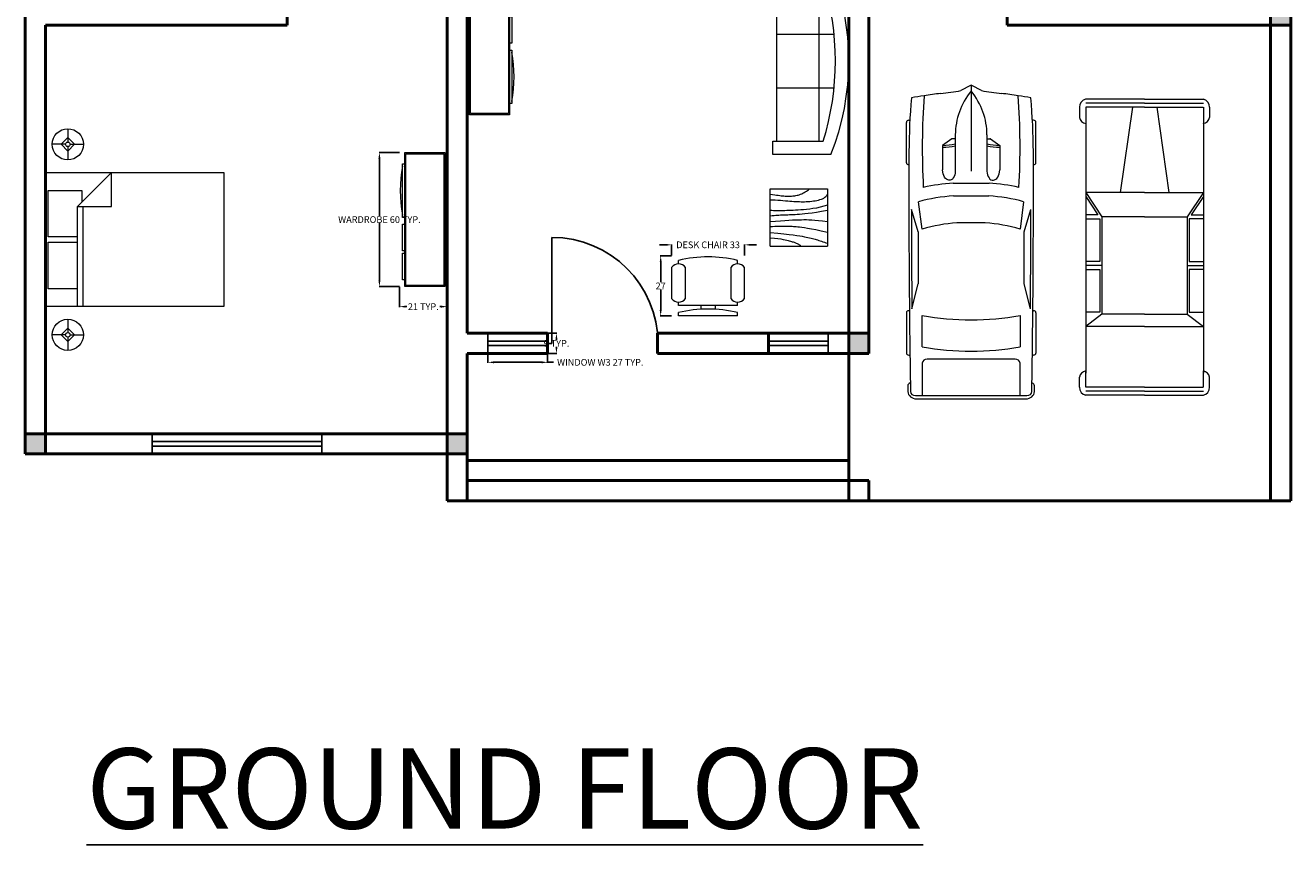
# Model space of a CAD drawing. Units: inches. Extents: x 13 to 1693, y -7 to 1519.
# Tile 1 of 10: x 116 to 683, y -7 to 360. Entities that reach past the tile are written whole.
import ezdxf

# ---------------------------------------------------------------- set-up
doc = ezdxf.new("R2010")
doc.units = ezdxf.units.IN
doc.header["$MEASUREMENT"] = 0
for name, color, linetype, lineweight in [('A-ANNO-DIMS', 2, 'Continuous', 18), ('A-ANNO-TEXT', 7, 'Continuous', 25), ('A-DOOR', 4, 'Continuous', 25), ('A-EQPM', 8, 'Continuous', 18), ('A-FURN', 8, 'Continuous', 18), ('A-GLAZ', 4, 'Continuous', 25), ('A-WALL', 7, 'Continuous', 50), ('A-WALL-PATT', 8, 'Continuous', 13)]:
    doc.layers.add(name, color=color, linetype=linetype, lineweight=lineweight)
doc.styles.get("Standard").update_dxf_attribs({"font": 'arial.ttf'})
doc.dimstyles.get("Standard").update_dxf_attribs({"dimtxt": 3, "dimasz": 2.68, "dimexe": 0.18, "dimexo": 0.0625, "dimgap": 0.09, "dimtad": 0, "dimtih": 1, "dimtoh": 1, "dimdec": 0, "dimzin": 0, "dimdsep": 46, "dimlunit": 3, "dimtxsty": 'Standard', "dimcen": 0.09, "dimadec": 0, "dimazin": 0, "dimtfac": 1, "dimtdec": 0, "dimtofl": 0, "dimtmove": 0, "dimatfit": 3, "dimfxl": 1, "dimtolj": 1, "dimtzin": 0, "dimarcsym": 0})

# ---------------------------------------------------------------- blocks, each defined once
blk = doc.blocks.new('Chair - Desk')
for p, q in [((-8.5, 0), (-8.5, -1)), ((-8.5, 0), (8.5, 0)), ((8.5, 0), (8.5, -1)), ((-8.5, -3), (-8.5, -4)), ((-8.5, -3), (8.5, -3)), ((-2, -3), (-2, -1.9355)), ((2, -1.9576), (2, -3)), ((8.5, -3), (8.5, -4)), ((-10.5, -5), (-10.5, -14)), ((-6.5, -14), (-6.5, -5)), ((6.5, -5), (6.5, -14)), ((10.5, -14), (10.5, -5)), ((-8.5, -15), (-8.5, -16)), ((8.5, -15), (8.5, -16))]:
    blk.add_line(p, q)
for centre, radius, start, end in [((0, 34.625), 36.625, 256.5803, 283.4197), ((-8.5, -6.5), 2.5, 36.8699, 143.1301), ((8.5, -6.5), 2.5, 36.8699, 143.1301), ((-8.5, -12.5), 2.5, 216.8699, 323.1301), ((8.5, -12.5), 2.5, 216.8699, 323.1301), ((0, 19.625), 36.625, 256.5803, 283.4197)]:
    blk.add_arc(centre, radius, start, end)
blk = doc.blocks.new('Sofa - Roundback 7 ft.')
for p, q in [((-12.00002, -32.4421), (-12.00003, -6.5971)), ((11.99997, -32.4421), (11.99998, -6.5971)), ((-36.000027, -34), (-36.000027, -11.4696)), ((-35.999844, -13.3819), (35.9998, -13.3819)), ((35.99998, -34), (35.99998, -11.4696)), ((-36.000027, -32.4421), (35.99998, -32.4421))]:
    blk.add_line(p, q)
for points in [[(-36.000027, -34), (-42.000027, -34), (-42.000027, -8)], [(41.99998, -8), (41.99998, -34), (35.99998, -34)]]:
    blk.add_lwpolyline(points)
for centre, radius, start, end in [((0, -114.25), 114.25, 68.43141, 111.5686), ((-0.00001, -127.1968), 121.1968, 72.72033, 107.2797)]:
    blk.add_arc(centre, radius, start, end)
blk = doc.blocks.new('Entertainment Center')
for p, q in [((-4, 0), (-5, -1)), ((4, 0), (-4, 0)), ((5, -1), (4, 0)), ((-17, -19), (-17, -1)), ((-17, -1), (43, -1)), ((-16.5, -18.5), (-16.5, -1.5)), ((-16.5, -1.5), (42.5, -1.5)), ((42.5, -1.5), (42.5, -18.5)), ((43, -1), (43, -19)), ((43, -19), (-17, -19)), ((42.5, -18.5), (-16.5, -18.5)), ((-12, -20), (-12, -19)), ((12, -20), (-12, -20)), ((12, -19), (12, -20)), ((15, -20), (15, -19)), ((27, -20), (15, -20)), ((27, -19), (27, -20)), ((28, -20), (28, -19)), ((40, -20), (28, -20)), ((40, -19), (40, -20))]:
    blk.add_line(p, q)
blk.add_arc((0, 40), 61, 259.6111, 280.3889)
blk = doc.blocks.new('Bed - Queen')
for p, q in [((0, -80.00003), (0, 0)), ((0, 0), (59.99999, 0)), ((59.99999, 0), (59.99999, -80.00003)), ((7.99999, -1.2), (28.79998, -1.2)), ((7.99999, -14.4), (7.99999, -1.2)), ((28.79998, -1.2), (28.79998, -14.4)), ((31.19999, -1.2), (51.99999, -1.2)), ((31.19999, -14.4), (31.19999, -1.2)), ((51.99999, -1.2), (51.99999, -16.4)), ((0, -14.4), (44.8, -14.4)), ((44.8, -16.8), (0, -16.8)), ((59.99999, -29.6), (44.8, -14.4)), ((44.8, -14.4), (44.8, -29.6)), ((51.99999, -16.4), (46.79936, -16.4)), ((44.8, -29.6), (59.99999, -29.6)), ((59.99999, -80.00003), (0, -80.00003))]:
    blk.add_line(p, q)
blk = doc.blocks.new('Lamp - Table')
for p, q in [((0, 7), (0, 1)), ((-1, 0), (-7, 0)), ((0, 3), (-3, 0)), ((-3, 0), (0, -3)), ((3, 0), (0, 3)), ((0, -3), (3, 0)), ((1, 0), (7, 0)), ((0, -1), (0, -7))]:
    blk.add_line(p, q)
for radius in [7, 1]:
    blk.add_circle((0, 0), radius)
blk = doc.blocks.new('Table - Square Woodgrain 42 x 42 in.')
blk.add_line((0, -42), (42, -42))
for points in [[(0, -4), (1.704, -4.2172), (3.2358, -4.4188), (4.615, -4.604), (5.8615, -4.7721), (6.9951, -4.9224), (8.0357, -5.0541), (9.0031, -5.1667), (9.9171, -5.2594), (10.7951, -5.3316), (11.6445, -5.3836), (12.4702, -5.4157), (13.277, -5.4283), (14.0698, -5.4217), (14.8535, -5.3964), (15.6331, -5.3526), (16.4133, -5.2908), (17.1986, -5.2103), (17.9913, -5.1062), (18.793, -4.9727), (19.6056, -4.8038), (20.4307, -4.5937), (21.2701, -4.3365), (22.1256, -4.0262), (22.9989, -3.6571), (23.888, -3.2272), (24.7756, -2.7516), (25.6408, -2.2491), (26.4624, -1.7387), (27.2195, -1.2395), (27.891, -0.7703), (28.456, -0.3501), (28.8934, 0.002)], [(0, -42), (0, 0), (42, 0), (42, -42)], [(0, -8), (1.8203, -8.1001), (3.6741, -8.2149), (5.5411, -8.3408), (7.4011, -8.4741), (9.2339, -8.6112), (11.0193, -8.7484), (12.7371, -8.8821), (14.3671, -9.0086), (15.8954, -9.1246), (17.3337, -9.2278), (18.6997, -9.3159), (20.0116, -9.387), (21.2871, -9.4389), (22.5442, -9.4696), (23.8008, -9.477), (25.0749, -9.459), (26.3791, -9.4137), (27.7049, -9.3403), (29.0383, -9.2382), (30.3655, -9.1068), (31.6728, -8.9455), (32.9461, -8.7535), (34.1717, -8.5304), (35.3358, -8.2756), (36.4268, -7.9863), (37.443, -7.6521), (38.3849, -7.2603), (39.253, -6.7986), (40.048, -6.2542), (40.7705, -5.6147), (41.421, -4.8674), (42, -4)], [(42, -12), (39.1784, -12.8621), (36.4519, -13.5654), (33.8246, -14.1294), (31.3004, -14.5731), (28.8832, -14.9161), (26.577, -15.1775), (24.3858, -15.3768), (22.3136, -15.5332), (20.3622, -15.6632), (18.5254, -15.7718), (16.7947, -15.8612), (15.1618, -15.9338), (13.6183, -15.9916), (12.1558, -16.0369), (10.7659, -16.0718), (9.4403, -16.0987), (8.1703, -16.1191), (6.9461, -16.1325), (5.7577, -16.1377), (4.595, -16.1335), (3.4479, -16.1188), (2.3064, -16.0924), (1.1604, -16.0532), (0, -16)], [(42, -16), (37.6529, -16.7365), (33.8802, -17.329), (30.6179, -17.7961), (27.8015, -18.1561), (25.3668, -18.4275), (23.2497, -18.6288), (21.3859, -18.7785), (19.7111, -18.8949), (18.1693, -18.9939), (16.7375, -19.0795), (15.401, -19.1534), (14.1449, -19.217), (12.9544, -19.2717), (11.8148, -19.3191), (10.7113, -19.3606), (9.6291, -19.3976), (8.5534, -19.4323), (7.47, -19.4689), (6.3643, -19.5122), (5.222, -19.5672), (4.0288, -19.6386), (2.7703, -19.7313), (1.4321, -19.8501), (0, -20)], [(0, -24), (3.9243, -23.6805), (7.4766, -23.4138), (10.6891, -23.1954), (13.5943, -23.0205), (16.2247, -22.8847), (18.6125, -22.7832), (20.7903, -22.7116), (22.7903, -22.6651), (24.6563, -22.642), (26.4764, -22.6507), (28.35, -22.7024), (30.3766, -22.8084), (32.6555, -22.98), (35.2861, -23.2283), (38.3678, -23.5645), (42, -24)], [(42, -32), (37.392, -31.017), (33.4585, -30.2231), (30.1291, -29.5949), (27.3334, -29.109), (25.0009, -28.742), (23.0612, -28.4707), (21.4439, -28.2716), (20.0786, -28.1215), (18.8998, -28.0002), (17.8609, -27.9014), (16.9206, -27.8219), (16.0371, -27.7588), (15.1691, -27.709), (14.2748, -27.6693), (13.3128, -27.6368), (12.2415, -27.6083), (11.0295, -27.5824), (9.6867, -27.5643), (8.233, -27.5608), (6.6884, -27.5787), (5.0728, -27.6248), (3.4062, -27.7058), (1.7086, -27.8286), (0, -28)], [(0, -32), (5.4026, -32.5358), (9.9494, -33.019), (13.7424, -33.4553), (16.8834, -33.8505), (19.4743, -34.2106), (21.6171, -34.5413), (23.4136, -34.8486), (24.9657, -35.1382), (26.3614, -35.4156), (27.6332, -35.6841), (28.7995, -35.9467), (29.8788, -36.2064), (30.8897, -36.4661), (31.8507, -36.7288), (32.7802, -36.9973), (33.6968, -37.2747), (34.6175, -37.5635), (35.5531, -37.8651), (36.5128, -38.1805), (37.506, -38.5108), (38.5421, -38.8568), (39.6302, -39.2197), (40.7797, -39.6004), (42, -40)], [(0, -36), (3.0098, -36.2857), (5.5354, -36.5643), (7.6368, -36.8359), (9.374, -37.1009), (10.807, -37.3597), (11.9957, -37.6126), (13.0002, -37.8599), (13.8804, -38.102), (14.6874, -38.3393), (15.4365, -38.5729), (16.1338, -38.8041), (16.7858, -39.0341), (17.3987, -39.264), (17.9787, -39.4952), (18.5322, -39.7288), (19.0655, -39.9662), (19.5832, -40.2081), (20.0842, -40.4544), (20.5657, -40.7046), (21.0249, -40.9581), (21.459, -41.2144), (21.8653, -41.4731), (22.2409, -41.7335), (22.5831, -41.9951)]]:
    blk.add_lwpolyline(points)
blk = doc.blocks.new('*U25')
for p, q in [((46.55, 38.89), (22.35, 38.89)), ((136.7, 38.89), (160.9, 38.89)), ((21.1, 37.41), (21.1, 36.83)), ((47.8, 37.39), (47.8, 37.41)), ((70.03, 31.54), (86.41, 29.35)), ((87.99, 31.87), (74.76, 35.92)), ((134.31, 35.6), (119.29, 31.78)), ((135.45, 37.07), (135.45, 37.41)), ((162.15, 37.41), (162.15, 36.77)), ((186.47, -33.5), (186.47, 33.5)), ((188.4, -32.76), (188.4, 32.76)), ((138.42, 29.35), (157.25, 29.35)), ((164.52, 26.39), (164.52, -26.39)), ((186.47, 29.35), (167.01, 29.35)), ((32.27, 11.63), (36.13, 17.17)), ((36.13, 17.17), (50.94, 17.17)), ((29.77, 9.51), (51.68, 9.51)), ((32.12, 9.51), (32.12, 11.15)), ((58.92, -10.77), (58.92, 10.77)), ((66.55, -10.53), (66.55, 10.53)), ((82.74, 8.5), (82.74, -8.5)), ((186.47, -10.53), (186.47, 10.53)), ((3.27, 6.13), (0.1, 0.41)), ((0, 0), (51.68, 0)), ((0.1, -0.41), (3.27, -6.13)), ((29.77, -9.51), (51.68, -9.51)), ((32.12, -9.51), (32.12, -11.15)), ((32.27, -11.63), (36.13, -17.17)), ((36.13, -17.17), (50.94, -17.17)), ((86.41, -29.35), (70.03, -31.54)), ((157.25, -29.35), (138.42, -29.35)), ((167.01, -29.35), (186.47, -29.35)), ((21.1, -37.41), (21.1, -36.83)), ((47.8, -37.39), (47.8, -37.41)), ((87.99, -31.87), (74.76, -35.92)), ((134.31, -35.6), (119.29, -31.78)), ((135.45, -37.07), (135.45, -37.41)), ((162.15, -37.41), (162.15, -36.77)), ((46.55, -38.89), (22.35, -38.89)), ((136.7, -38.89), (160.9, -38.89))]:
    blk.add_line(p, q)
for centre, major_axis, ratio, start_param, end_param in [((22.35, 37.41), (0, -1.48), 0.842304, 3.141593, 4.712389), ((46.55, 37.41), (0, 1.48), 0.842304, -1.570796, 0), ((136.7, 37.41), (0, -1.48), 0.842304, 3.141593, 4.712389), ((160.9, 37.41), (0, 1.48), 0.842304, -1.570796, 0), ((180.63, 35.84), (0, 2.22), 0.842304, -0.013017, 1.249894), ((64.48, -10556.36), (0, 10595.31), 0.842304, -0.013397, -0.013017), ((266.03, -27.52), (0, 313.31), 0.842304, 1.367076, 1.39176), ((41.19, -490.86), (0, 528.23), 0.842304, 0.00281, 0.075598), ((64.48, -10555.62), (0, 10593.03), 0.842304, -0.013397, 0.002797), ((135.29, 5.39), (0, 81.77), 0.842304, 1.245306, 1.50788), ((64.48, -10555.62), (0, -10591.55), 0.842304, 3.133765, 3.140441), ((95.79, -3666.35), (0, -3698.24), 0.842304, 3.134049, 3.144098), ((183.98, 33.5), (0, -2.96), 0.842304, 1.570796, 3.128196), ((183.98, 32.76), (0, -5.25), 0.842304, 1.570796, 3.128196), ((259.18, -27.52), (0, -305.3), 0.842304, 4.528606, 4.561838), ((37.47, -593.96), (0, -623.33), 0.842304, 3.096046, 3.200911), ((134.4, 5.39), (0, -89.78), 0.842304, 4.449482, 4.652344), ((149.6, 2.8), (0, -79.58), 0.842304, 4.372215, 4.640744), ((17.08, 0), (0, 147.02), 0.842304, 4.511394, 4.913384), ((35.91, 0), (0, 147.02), 0.842304, 4.511394, 4.913384), ((167.01, 26.39), (0, 2.96), 0.842304, 0, 1.570796), ((-204.49, 52.4), (0, -250.96), 0.842304, 1.385369, 1.434372), ((13.04, 17.01), (0, 27.42), 0.842304, 4.435146, 4.718221), ((14.2, 17.01), (0, 27.42), 0.842304, 4.435146, 4.718221), ((50.79, 13.34), (6.34, -0.36), 0.603834, -1.395552, 1.581315), ((29.77, -46.66), (0, 56.17), 0.842304, 0, 0.590319), ((32.75, 11.15), (0, 0.74), 0.842304, 0.879714, 1.570796), ((0.62, 0), (0, -0.74), 0.842304, 4.131459, 5.293319), ((-204.49, -52.4), (0, 250.96), 0.842304, -1.434372, -1.385369), ((29.77, 46.66), (0, 56.17), 0.842304, 2.551274, 3.141593), ((32.75, -11.15), (0, -0.74), 0.842304, 4.712389, 5.403472), ((13.04, -17.01), (0, -27.42), 0.842304, 1.564964, 1.848039), ((14.2, -17.01), (0, -27.42), 0.842304, 1.564964, 1.848039), ((134.4, -5.39), (0, -89.78), 0.842304, -1.510751, -1.307889), ((135.29, -5.39), (0, -81.77), 0.842304, -1.50788, -1.245306), ((149.6, -2.8), (0, -79.58), 0.842304, -1.499151, -1.230623), ((259.18, 27.52), (0, 305.3), 0.842304, 1.721348, 1.754579), ((266.03, 27.52), (0, 313.31), 0.842304, 1.749832, 1.774517), ((37.47, 593.96), (0, -623.33), 0.842304, -0.059319, 0.045547), ((167.01, -26.39), (0, -2.96), 0.842304, 4.712389, 6.283185), ((41.19, 490.86), (0, -528.23), 0.842304, -0.075598, -0.00281), ((22.35, -37.41), (0, 1.48), 0.842304, 1.570796, 3.141593), ((64.48, 10555.62), (0, 10593.03), 0.842304, 3.138796, 3.15499), ((46.55, -37.41), (0, -1.48), 0.842304, 0, 1.570796), ((64.48, 10555.62), (0, -10591.55), 0.842304, 0.001152, 0.007828), ((95.79, 3666.35), (0, -3698.24), 0.842304, -0.002505, 0.007544), ((136.7, -37.41), (0, -1.48), 0.842304, -1.570796, 0), ((160.9, -37.41), (0, 1.48), 0.842304, 3.141593, 4.712389), ((180.63, -35.84), (0, -2.22), 0.842304, -1.249894, 0.013017), ((64.48, 10556.36), (0, 10595.31), 0.842304, 3.15461, 3.15499), ((183.98, -33.5), (0, 2.96), 0.842304, 3.15499, 4.712389), ((183.98, -32.76), (0, -5.25), 0.842304, 0.013397, 1.570796)]:
    blk.add_ellipse(centre, major_axis=major_axis, ratio=ratio, start_param=start_param, end_param=end_param)
at = {"extrusion": (0, 0, -1)}
blk.add_ellipse((50.79, -13.34), major_axis=(6.34, 0.36), ratio=0.603834, start_param=-1.395552, end_param=1.581315, dxfattribs=at)
blk = doc.blocks.new('*U26')
for p, q in [((5.44, 42.31), (12.12, 42.31)), ((189.69, 42.31), (183.01, 42.31)), ((0.1, -0.41), (0.1, 38.35)), ((2.77, -0.41), (2.77, 38.31)), ((5.44, -0.41), (5.44, 38.24)), ((5.45, 38.31), (16.12, 38.31)), ((16.12, 38.31), (180.34, 38.31)), ((61.52, -0.41), (61.52, 38.31)), ((61.52, 38.31), (77.54, 27.62)), ((64.19, 38.31), (76.2, 30.29)), ((76.2, 30.29), (76.2, 38.31)), ((78.87, 38.31), (78.87, 28.96)), ((106.91, 28.96), (106.91, 38.31)), ((109.58, 27.62), (109.58, 38.31)), ((112.25, 38.31), (112.25, 28.96)), ((140.29, 28.96), (140.29, 38.31)), ((141.62, 27.62), (149.64, 38.31)), ((149.64, -0.41), (149.64, 38.31)), ((189.69, 38.31), (179.01, 38.31)), ((189.69, -0.41), (189.69, 38.24)), ((192.36, -0.41), (192.36, 38.31)), ((195.03, -0.41), (195.03, 38.35)), ((77.54, 27.62), (141.62, 27.62)), ((77.54, -0.41), (77.54, 27.62)), ((78.87, 28.96), (106.91, 28.96)), ((112.25, 28.96), (140.29, 28.96)), ((141.62, -0.41), (141.62, 27.62)), ((5.44, 7.6), (61.52, 15.61)), ((0.1, -0.42), (0.1, -39.18)), ((2.77, -0.41), (2.77, -39.13)), ((5.44, -0.42), (5.44, -39.07)), ((61.52, -0.41), (61.52, -39.13)), ((77.54, -0.41), (77.54, -28.45)), ((141.62, -0.41), (141.62, -28.45)), ((149.64, -0.41), (149.64, -39.13)), ((189.69, -0.42), (189.69, -39.07)), ((192.36, -0.41), (192.36, -39.13)), ((195.03, -0.42), (195.03, -39.18)), ((5.44, -8.42), (61.52, -16.43)), ((61.52, -39.13), (77.54, -28.45)), ((64.19, -39.13), (76.2, -31.12)), ((76.2, -31.12), (76.2, -39.13)), ((77.54, -28.45), (141.62, -28.45)), ((78.87, -39.13), (78.87, -29.79)), ((78.87, -29.79), (106.91, -29.79)), ((106.91, -29.79), (106.91, -39.13)), ((109.58, -28.45), (109.58, -39.13)), ((112.25, -29.79), (140.29, -29.79)), ((112.25, -39.13), (112.25, -29.79)), ((140.29, -29.79), (140.29, -39.13)), ((141.62, -28.45), (149.64, -39.13)), ((5.45, -39.13), (16.12, -39.13)), ((16.12, -39.13), (180.34, -39.13)), ((189.69, -39.13), (179.01, -39.13)), ((5.44, -43.14), (12.12, -43.14)), ((189.69, -43.14), (183.01, -43.14))]:
    blk.add_line(p, q)
for centre, radius, start, end in [((5.06, 37.26), 5.06, 85.64554, 168.0943), ((11.45, 37.64), 4.72, 8.13011, 81.86996), ((183.68, 37.64), 4.72, 98.13004, 171.8699), ((190.07, 37.26), 5.06, 11.90574, 94.35446), ((5.06, -38.09), 5.06, 191.9057, 274.3545), ((11.45, -38.46), 4.72, 278.13, 351.8699), ((183.68, -38.46), 4.72, 188.1301, 261.87), ((190.07, -38.09), 5.06, 265.6455, 348.0943)]:
    blk.add_arc(centre, radius, start, end)
blk = doc.blocks.new('WIN-76')
for p, q in [((0, 9), (0, 0)), ((76.02, 9), (76.02, 0)), ((0, 5.5), (76.02, 5.5)), ((0, 3.5), (76.02, 3.5))]:
    blk.add_line(p, q)
blk = doc.blocks.new('WIN-27-SIDE')
for p, q in [((0, 9), (0, 0)), ((0, 5.5), (26.68, 5.5)), ((0, 3.5), (26.68, 3.5))]:
    blk.add_line(p, q)
blk = doc.blocks.new('DOOR-48')
for p, q in [((2, 0), (2, 47.5)), ((0, 0), (2, 0))]:
    blk.add_line(p, q)
blk.add_arc((2, 0), 47.5, 0, 90)
blk = doc.blocks.new('*D40')
at = {"layer": 'A-ANNO-DIMS', "color": 0, "lineweight": -2, "transparency": 16777216}
for p, q in [((284.06, 303.11), (274.94, 303.11)), ((275.12, 300.43), (275.12, 274.75)), ((275.12, 245.79), (275.12, 271.46)), ((284.06, 243.11), (274.94, 243.11))]:
    blk.add_line(p, q, dxfattribs=at)
at = {"layer": 'A-ANNO-DIMS', "color": 0, "transparency": 16777216}
for points in [[(274.67, 300.43), (275.57, 300.43), (275.12, 303.11)], [(274.67, 245.79), (275.57, 245.79), (275.12, 243.11)]]:
    blk.add_solid(points, dxfattribs=at)
at = {"layer": 'Defpoints', "color": 0, "transparency": 16777216}
for p in [(284.12, 303.11), (275.12, 243.11), (284.12, 243.11)]:
    blk.add_point(p, dxfattribs=at)
at = {"layer": 'A-ANNO-DIMS', "color": 0, "transparency": 16777216, "insert": (275.12, 273.11), "char_height": 3, "attachment_point": 5}
blk.add_mtext('\\A1;WARDROBE 60 TYP.', dxfattribs=at)
blk = doc.blocks.new('*D41')
at = {"layer": 'A-ANNO-DIMS', "color": 0, "lineweight": -2, "transparency": 16777216}
for p, q in [((284.12, 243.04), (284.12, 233.93)), ((305.45, 243.04), (305.45, 233.93)), ((286.8, 234.11), (287.37, 234.11)), ((302.77, 234.11), (302.2, 234.11))]:
    blk.add_line(p, q, dxfattribs=at)
at = {"layer": 'A-ANNO-DIMS', "color": 0, "transparency": 16777216}
for points in [[(286.8, 234.55), (286.8, 233.66), (284.12, 234.11)], [(302.77, 234.55), (302.77, 233.66), (305.45, 234.11)]]:
    blk.add_solid(points, dxfattribs=at)
at = {"layer": 'Defpoints', "color": 0, "transparency": 16777216}
for p in [(284.12, 243.11), (305.45, 243.11), (305.45, 234.11)]:
    blk.add_point(p, dxfattribs=at)
at = {"layer": 'A-ANNO-DIMS', "color": 0, "transparency": 16777216, "insert": (294.79, 234.11), "char_height": 3, "attachment_point": 5}
blk.add_mtext('\\A1;21 TYP.', dxfattribs=at)
blk = doc.blocks.new('*D48')
at = {"layer": 'A-ANNO-DIMS', "color": 0, "lineweight": -2, "transparency": 16777216}
for p, q in [((323.77, 213.09), (323.77, 208.97)), ((350.45, 213.09), (350.45, 208.97)), ((326.45, 209.15), (347.77, 209.15)), ((350.45, 209.15), (353.13, 209.15))]:
    blk.add_line(p, q, dxfattribs=at)
at = {"layer": 'A-ANNO-DIMS', "color": 0, "transparency": 16777216}
for points in [[(326.45, 209.6), (326.45, 208.7), (323.77, 209.15)], [(347.77, 209.6), (347.77, 208.7), (350.45, 209.15)]]:
    blk.add_solid(points, dxfattribs=at)
at = {"layer": 'Defpoints', "color": 0, "transparency": 16777216}
for p in [(323.77, 213.15), (350.45, 213.15), (350.45, 209.15)]:
    blk.add_point(p, dxfattribs=at)
at = {"layer": 'A-ANNO-DIMS', "color": 0, "transparency": 16777216, "insert": (374.09, 209.15), "char_height": 3, "attachment_point": 5}
blk.add_mtext('\\A1;WINDOW W3 27 TYP.', dxfattribs=at)
blk = doc.blocks.new('*D49')
at = {"layer": 'A-ANNO-DIMS', "color": 0, "lineweight": -2, "transparency": 16777216}
for p, q in [((350.52, 222.15), (354.64, 222.15)), ((354.46, 219.47), (354.46, 219.27)), ((354.46, 215.83), (354.46, 216.03)), ((350.52, 213.15), (354.64, 213.15))]:
    blk.add_line(p, q, dxfattribs=at)
at = {"layer": 'A-ANNO-DIMS', "color": 0, "transparency": 16777216}
for points in [[(354.01, 219.47), (354.9, 219.47), (354.46, 222.15)], [(354.01, 215.83), (354.9, 215.83), (354.46, 213.15)]]:
    blk.add_solid(points, dxfattribs=at)
at = {"layer": 'Defpoints', "color": 0, "transparency": 16777216}
for p in [(350.45, 222.15), (354.46, 222.15), (350.45, 213.15)]:
    blk.add_point(p, dxfattribs=at)
at = {"layer": 'A-ANNO-DIMS', "color": 0, "transparency": 16777216, "insert": (354.46, 217.65), "char_height": 3, "attachment_point": 5}
blk.add_mtext('\\A1;9 TYP.', dxfattribs=at)
blk = doc.blocks.new('*D68')
at = {"layer": 'A-ANNO-DIMS', "color": 0, "lineweight": -2, "transparency": 16777216}
for p, q in [((403.38, 261.8), (400.7, 261.8)), ((406.06, 256.96), (406.06, 261.98)), ((438.75, 256.96), (438.75, 261.98)), ((441.43, 261.8), (444.11, 261.8))]:
    blk.add_line(p, q, dxfattribs=at)
at = {"layer": 'A-ANNO-DIMS', "color": 0, "transparency": 16777216}
for points in [[(403.38, 262.24), (403.38, 261.35), (406.06, 261.8)], [(441.43, 262.24), (441.43, 261.35), (438.75, 261.8)]]:
    blk.add_solid(points, dxfattribs=at)
at = {"layer": 'Defpoints', "color": 0, "transparency": 16777216}
for p in [(406.06, 261.8), (406.06, 256.89), (438.75, 256.89)]:
    blk.add_point(p, dxfattribs=at)
at = {"layer": 'A-ANNO-DIMS', "color": 0, "transparency": 16777216, "insert": (422.41, 261.8), "char_height": 3, "attachment_point": 5}
blk.add_mtext('\\A1;DESK CHAIR 33', dxfattribs=at)
blk = doc.blocks.new('*D69')
at = {"layer": 'A-ANNO-DIMS', "color": 0, "lineweight": -2, "transparency": 16777216}
for p, q in [((405.99, 256.89), (400.97, 256.89)), ((401.15, 254.21), (401.15, 245)), ((401.15, 232.59), (401.15, 241.8)), ((405.99, 229.91), (400.97, 229.91))]:
    blk.add_line(p, q, dxfattribs=at)
at = {"layer": 'A-ANNO-DIMS', "color": 0, "transparency": 16777216}
for points in [[(400.71, 254.21), (401.6, 254.21), (401.15, 256.89)], [(400.71, 232.59), (401.6, 232.59), (401.15, 229.91)]]:
    blk.add_solid(points, dxfattribs=at)
at = {"layer": 'Defpoints', "color": 0, "transparency": 16777216}
for p in [(406.06, 256.89), (401.15, 229.91), (406.06, 229.91)]:
    blk.add_point(p, dxfattribs=at)
at = {"layer": 'A-ANNO-DIMS', "color": 0, "transparency": 16777216, "insert": (401.15, 243.4), "char_height": 3, "attachment_point": 5}
blk.add_mtext('\\A1;27', dxfattribs=at)

msp = doc.modelspace()

# ---------------------------------------------------------------- hatches: boundary and pattern name
at = {"layer": 'A-WALL-PATT'}
h = msp.add_hatch(color=256, dxfattribs=at)
h.dxf.hatch_style = 1
h.paths.add_polyline_path([(125.45, 735.15), (116.45, 735.15), (116.45, 726.15), (125.45, 726.15)])
h.paths.add_polyline_path([(125.45, 657.15), (116.45, 657.15), (116.45, 648.15), (125.45, 648.15)])
h.paths.add_polyline_path([(125.45, 498.15), (116.45, 498.15), (116.45, 489.15), (125.45, 489.15)])
h.paths.add_polyline_path([(125.45, 417.15), (116.45, 417.15), (116.45, 408.15), (125.45, 408.15)])
h.paths.add_polyline_path([(125.45, 177.15), (116.45, 177.15), (116.45, 168.15), (125.45, 168.15)])
h.paths.add_polyline_path([(314.45, 177.15), (305.45, 177.15), (305.45, 168.15), (314.45, 168.15)])
h.paths.add_polyline_path([(314.45, 417.15), (305.45, 417.15), (305.45, 408.15), (314.45, 408.15)])
h.paths.add_polyline_path([(314.45, 498.15), (305.45, 498.15), (305.45, 489.15), (314.45, 489.15)])
h.paths.add_polyline_path([(314.45, 657.15), (305.45, 657.15), (305.45, 648.15), (314.45, 648.15)])
h.paths.add_polyline_path([(314.45, 735.15), (305.45, 735.15), (305.45, 726.15), (314.45, 726.15)])
h = msp.add_hatch(color=256, dxfattribs=at)
h.dxf.hatch_style = 1
h.paths.add_polyline_path([(683.45, 735.15), (674.45, 735.15), (674.45, 726.15), (683.45, 726.15)])
h.paths.add_polyline_path([(683.45, 657.15), (674.45, 657.15), (674.45, 648.15), (683.45, 648.15)])
h.paths.add_polyline_path([(494.45, 498.15), (485.45, 498.15), (485.45, 489.15), (494.45, 489.15)])
h.paths.add_polyline_path([(683.45, 498.15), (674.45, 498.15), (674.45, 489.15), (683.45, 489.15)])
h.paths.add_polyline_path([(494.45, 222.15), (485.45, 222.15), (485.45, 213.15), (494.45, 213.15)])
h.paths.add_polyline_path([(683.45, 369.15), (674.45, 369.15), (674.45, 360.15), (683.45, 360.15)])

# ---------------------------------------------------------------- linework, layer by layer
at = {"layer": 'A-WALL'}
for p, q in [((116.45, 168.15), (116.45, 735.15)), ((683.45, 147.15), (683.45, 735.15)), ((305.45, 417.15), (305.45, 168.15)), ((314.45, 417.15), (314.45, 222.15)), ((485.45, 213.15), (485.45, 417.15)), ((494.45, 213.15), (494.45, 408.15)), ((556.41, 408.15), (556.41, 360.15)), ((233.77, 376.65), (233.77, 360.15)), ((125.45, 168.15), (125.45, 360.15)), ((233.77, 360.15), (125.45, 360.15)), ((674.45, 360.15), (556.41, 360.15)), ((674.45, 147.15), (674.45, 360.15)), ((314.45, 222.15), (350.45, 222.15)), ((350.45, 222.15), (350.45, 213.15)), ((449.45, 222.15), (399.74, 222.15)), ((399.74, 222.15), (399.74, 213.15)), ((449.45, 213.15), (449.45, 222.15)), ((449.45, 222.15), (494.45, 222.15)), ((314.45, 177.15), (314.45, 213.15)), ((314.45, 213.15), (350.45, 213.15)), ((314.45, 213.15), (314.45, 168.15)), ((449.45, 213.15), (399.74, 213.15)), ((449.45, 213.15), (494.45, 213.15)), ((485.45, 213.15), (485.45, 147.15)), ((116.45, 177.15), (314.45, 177.15)), ((116.45, 168.15), (314.45, 168.15)), ((305.45, 168.15), (305.45, 156.15)), ((314.45, 147.15), (314.45, 168.15)), ((485.45, 165.15), (314.45, 165.15)), ((305.45, 156.15), (305.45, 147.15)), ((485.45, 156.15), (314.45, 156.15)), ((485.45, 147.15), (485.45, 156.15)), ((485.45, 156.15), (494.45, 156.15)), ((494.45, 147.15), (494.45, 156.15)), ((305.45, 147.15), (314.45, 147.15)), ((485.45, 147.15), (314.45, 147.15)), ((485.45, 147.15), (494.45, 147.15)), ((494.45, 147.15), (683.45, 147.15))]:
    msp.add_line(p, q, dxfattribs=at)
msp.add_lwpolyline([(674.45, 369.15), (683.45, 369.15), (683.45, 360.15), (674.45, 360.15)], close=True, dxfattribs=at)

# ---------------------------------------------------------------- block references
at = {"layer": 'A-DOOR'}
msp.add_blockref('DOOR-48', (350.45, 217.65), dxfattribs=at)
at = {"layer": 'A-EQPM', "rotation": 270}
for name, p, xscale, yscale, zscale in [('*U25', (540.27, 333.32), 0.7458978152253524, 0.7458978152253524, 0.7458978152253524), ('*U26', (618.23, 327.14), 0.6807806149110928, 0.6807806149110928, 0.6807806149110928)]:
    msp.add_blockref(name, p, dxfattribs=dict(at, xscale=xscale, yscale=yscale, zscale=zscale))
at = {"layer": 'A-FURN'}
for name, p, rotation in [('Sofa - Roundback 7 ft.', (485.45, 344.21), 270), ('Entertainment Center', (314.45, 337.08), 90), ('Entertainment Center', (305.45, 286.11), 270), ('Bed - Queen', (125.45, 234.15), 90)]:
    msp.add_blockref(name, p, dxfattribs=dict(at, rotation=rotation))
for p in [(135.5, 306.83), (135.5, 221.45)]:
    msp.add_blockref('Lamp - Table', p, dxfattribs=at)
at = {"layer": 'A-FURN', "xscale": 0.6108650724074032, "yscale": 0.6108650724074032, "zscale": 0.6108650724074032}
msp.add_blockref('Table - Square Woodgrain 42 x 42 in.', (450.28, 286.91), dxfattribs=at)
at = {"layer": 'A-FURN', "xscale": 1.556931688025887, "yscale": 1.556931688025887, "zscale": 1.556931688025887, "rotation": 180}
msp.add_blockref('Chair - Desk', (422.41, 229.91), dxfattribs=at)
at = {"layer": 'A-GLAZ'}
for name, p in [('WIN-27-SIDE', (323.77, 213.15)), ('WIN-76', (173.34, 168.15))]:
    msp.add_blockref(name, p, dxfattribs=at)
at = {"layer": 'A-GLAZ', "rotation": 180}
msp.add_blockref('WIN-27-SIDE', (476.14, 222.15), dxfattribs=at)

# ---------------------------------------------------------------- texts
at = {"layer": 'A-ANNO-TEXT', "insert": (143.8, 36.23), "char_height": 36, "attachment_point": 1}
msp.add_mtext_dynamic_manual_height_columns('{\\LGROUND FLOOR}', width=444.8977, gutter_width=1, heights=[0], dxfattribs=at)

# ---------------------------------------------------------------- dimensions: what is measured, and where the dimension line sits
at = {"layer": 'A-ANNO-DIMS'}
for base, p1, p2, angle, text, picture, middle in [((275.12, 243.11), (284.12, 303.11), (284.12, 243.11), 270, 'WARDROBE <> TYP.', '*D40', (275.12, 273.11)), ((406.06, 261.8), (438.75, 256.89), (406.06, 256.89), 180, 'DESK CHAIR <>', '*D68', (422.41, 261.8)), ((354.46, 222.15), (350.45, 213.15), (350.45, 222.15), 90, '<> TYP.', '*D49', (354.46, 217.65))]:
    dim = msp.add_linear_dim(base=base, p1=p1, p2=p2, angle=angle, text=text, dimstyle='Standard', override={"dimdec": 0, "dimlfac": 1, "dimrnd": 0, "dimzin": 0, "dimdsep": 46, "dimlunit": 2}, dxfattribs=at)
    dim.commit()
    dim.dimension.update_dxf_attribs({"geometry": picture, "text_midpoint": middle})
dim = msp.add_linear_dim(base=(401.15, 229.91), p1=(406.06, 256.89), p2=(406.06, 229.91), angle=270, dimstyle='Standard', override={"dimdec": 0, "dimlfac": 1, "dimrnd": 0, "dimzin": 0, "dimdsep": 46, "dimlunit": 2}, dxfattribs=at)
dim.commit()
dim.dimension.update_dxf_attribs({"geometry": '*D69', "text_midpoint": (401.15, 243.4)})
for base, p1, p2, text, picture, middle in [((305.45, 234.11), (284.12, 243.11), (305.45, 243.11), '<> TYP.', '*D41', (294.79, 234.11)), ((350.45, 209.15), (323.77, 213.15), (350.45, 213.15), 'WINDOW W3 <> TYP.', '*D48', (374.09, 209.15))]:
    dim = msp.add_linear_dim(base=base, p1=p1, p2=p2, text=text, dimstyle='Standard', override={"dimdec": 0, "dimlfac": 1, "dimrnd": 0, "dimzin": 0, "dimdsep": 46, "dimlunit": 2}, dxfattribs=at)
    dim.commit()
    dim.dimension.update_dxf_attribs({"geometry": picture, "text_midpoint": middle})

doc.saveas('drawing.dxf')
